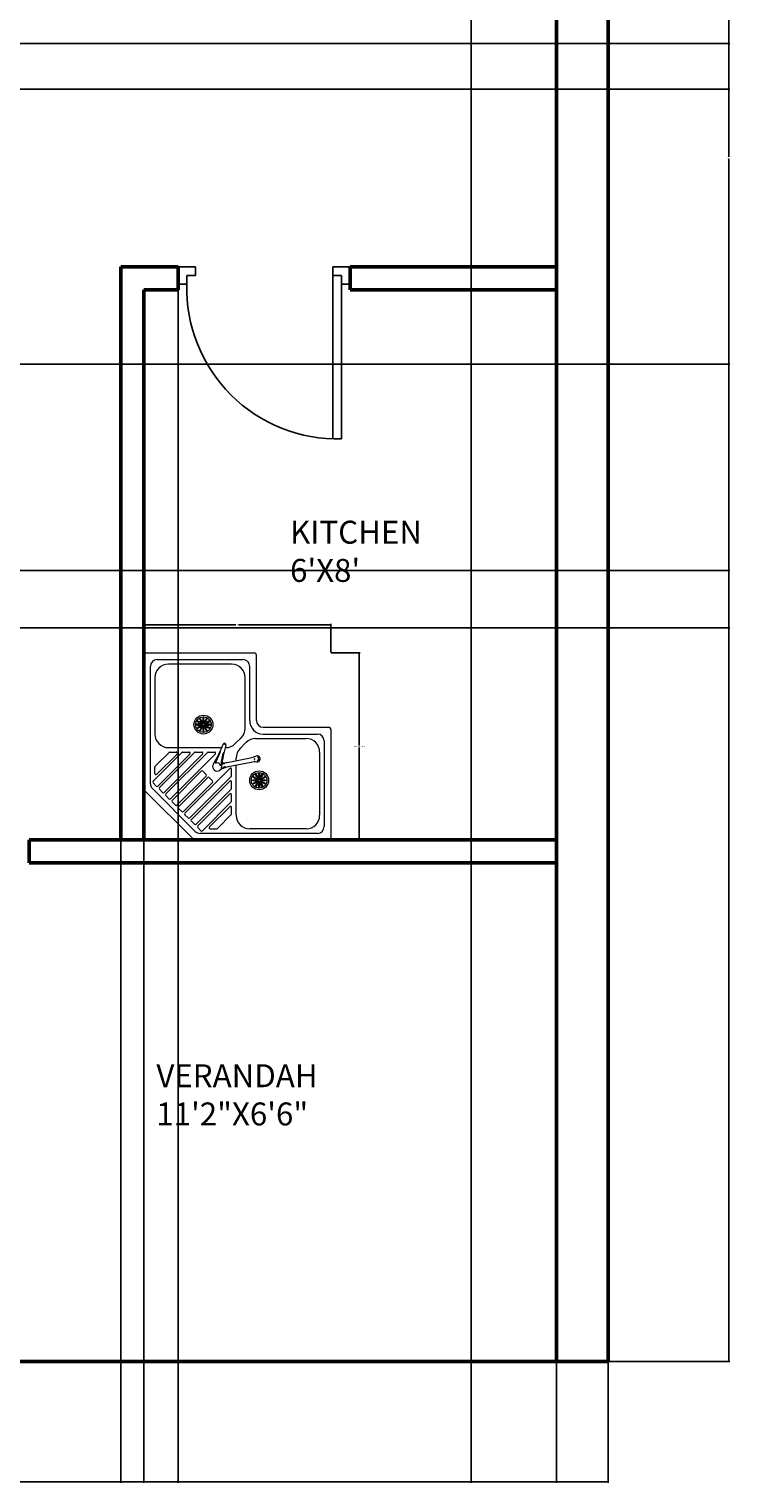
# Model space of a CAD drawing. Units: inches. Extents: x 1798 to 2141, y 1923 to 2386.
# Tile 4 of 9: x 2019 to 2141, y 1923 to 2177. Entities that reach past the tile are written whole.
import ezdxf

# ---------------------------------------------------------------- set-up
doc = ezdxf.new("R2010")
doc.units = ezdxf.units.IN
for name, color, linetype, lineweight in [('A-ANNO-DIMS', 2, 'Continuous', 18), ('A-AREA-IDEN', 7, 'Continuous', 25), ('A-FLOR-FIXT', 9, 'Continuous', 18), ('door', 40, 'Continuous', 25), ('wall', 4, 'Continuous', 50)]:
    doc.layers.add(name, color=color, linetype=linetype, lineweight=lineweight)
doc.styles.get("Standard").update_dxf_attribs({"font": 'arial.ttf'})
doc.dimstyles.get("Standard").update_dxf_attribs({"dimtxt": 0.18, "dimasz": 0.18, "dimexe": 0.18, "dimexo": 0.0625, "dimgap": 0.09, "dimtad": 0, "dimtih": 1, "dimtoh": 1, "dimdec": 4, "dimzin": 0, "dimdsep": 46, "dimtxsty": 'Standard', "dimcen": 0.09, "dimadec": 0, "dimazin": 0, "dimtfac": 1, "dimtdec": 4, "dimtofl": 0, "dimtmove": 0, "dimatfit": 3, "dimfxl": 1, "dimtolj": 1, "dimtzin": 0, "dimarcsym": 0})

# ---------------------------------------------------------------- blocks, each defined once
blk = doc.blocks.new('A$C4E531579')
for p, q in [((222.1, 827.1), (2.9, 607.9)), ((228.6, 791.2), (38.8, 601.4)), ((229.1, 830), (820, 830)), ((253.9, 788.2), (239.8, 774.1)), ((249.9, 800), (770, 800)), ((388.5, 660.7), (261, 788.2)), ((295.4, 780), (323.7, 780)), ((388.5, 717.2), (327.2, 778.5)), ((720, 780), (470, 780)), ((830, 820), (830, 340)), ((197.4, 731.6), (183.2, 717.5)), ((381.5, 512.2), (183.2, 710.4)), ((388.5, 547.5), (204.4, 731.6)), ((225.6, 759.9), (211.5, 745.8)), ((381.5, 568.7), (211.5, 738.7)), ((388.5, 604.1), (232.7, 759.9)), ((381.5, 625.3), (239.8, 767)), ((381.5, 681.9), (291.9, 771.5)), ((390, 713.7), (390, 685.4)), ((410, 720), (410, 483.9)), ((780, 440), (780, 720)), ((800, 770), (800, 390)), ((98.4, 632.6), (112.5, 646.8)), ((317.8, 448.5), (119.6, 646.8)), ((126.6, 660.9), (140.8, 675.1)), ((255.6, 524.9), (126.6, 653.9)), ((276.8, 546.1), (147.9, 675.1)), ((169.1, 703.4), (154.9, 689.2)), ((283.9, 553.2), (154.9, 682.1)), ((305.1, 574.4), (176.1, 703.4)), ((390, 657.1), (390, 628.8)), ((0, 10), (0, 600.9)), ((30, 60), (30, 580.1)), ((41.8, 576.1), (55.9, 590.2)), ((204.7, 448.5), (63, 590.2)), ((70.1, 604.4), (84.2, 618.5)), ((225.9, 441.5), (70.1, 597.3)), ((261.3, 448.5), (91.3, 618.5)), ((282.5, 441.5), (98.4, 625.6)), ((390, 600.6), (390, 572.3)), ((169.3, 441.5), (41.8, 569)), ((50, 534.6), (50, 506.3)), ((148.1, 448.5), (58.5, 538.1)), ((262.7, 524.9), (276.8, 539)), ((305.1, 567.3), (291, 553.2)), ((390, 544), (390, 515.7)), ((112.8, 441.5), (51.5, 502.8)), ((344.7, 353.4), (324.5, 455.5)), ((344.5, 460.1), (364.9, 357.1)), ((410, 468.8), (410, 466.1)), ((110, 420), (331.5, 420)), ((116.3, 440), (144.6, 440)), ((172.9, 440), (201.2, 440)), ((229.4, 440), (257.7, 440)), ((286, 440), (314.3, 440)), ((352.4, 420), (363.9, 420)), ((406.4, 402.4), (432.4, 376.4)), ((427.6, 423.6), (453.6, 397.6)), ((50, 110), (50, 360)), ((450, 333.9), (450, 110)), ((496.1, 380), (720, 380)), ((530, 360), (770, 360)), ((530, 330), (820, 330)), ((470, 300), (470, 60)), ((500, 300), (500, 10)), ((440, 30), (60, 30)), ((390, 50), (110, 50)), ((490, 0), (10, 0))]:
    blk.add_line(p, q)
for centre, radius in [((511.9, 565), 41.9), ((511.9, 565), 34.4), ((511.9, 565), 5.37), ((265, 318.1), 41.9), ((265, 318.1), 34.4), ((265, 318.1), 5.37)]:
    blk.add_circle(centre, radius)
for centre, radius, start, end in [((229.1, 820), 10, 90, 135), ((249.9, 770), 30, 90, 135), ((243.3, 770.5), 5, 135, 225), ((257.5, 784.7), 5, 45, 135), ((295.4, 775), 5, 90, 225), ((323.7, 775), 5, 45, 90), ((470, 720), 60, 90, 180), ((720, 720), 60, 0, 90), ((770, 770), 30, 0, 90), ((820, 820), 10, 0, 90), ((186.7, 714), 5, 135, 225), ((200.9, 728.1), 5, 45, 135), ((215, 742.2), 5, 135, 225), ((229.2, 756.4), 5, 45, 135), ((385, 713.7), 5, 0, 45), ((116, 643.3), 5, 45, 135), ((130.2, 657.4), 5, 135, 225), ((144.3, 671.5), 5, 45, 135), ((158.5, 685.7), 5, 135, 225), ((172.6, 699.8), 5, 45, 135), ((385, 685.4), 5, 225, 0), ((385, 657.1), 5, 0, 45), ((10, 600.9), 10, 135, 180), ((60, 580.1), 30, 135, 180), ((59.5, 586.7), 5, 45, 135), ((73.6, 600.8), 5, 135, 225), ((87.8, 615), 5, 45, 135), ((101.9, 629.1), 5, 135, 225), ((385, 628.8), 5, 225, 0), ((385, 600.6), 5, 0, 45), ((45.3, 572.5), 5, 135, 225), ((55, 534.6), 5, 45, 180), ((259.2, 528.4), 5, 225, 315), ((273.3, 542.6), 5, 315, 45), ((287.4, 556.7), 5, 225, 315), ((301.6, 570.8), 5, 315, 45), ((325.6, 504.4), 20, 52.72293, 268.78568), ((583, 916.9), 466.4, 238.27092, 250.20216), ((385, 572.3), 5, 225, 0), ((385, 515.7), 5, 225, 0), ((385, 544), 5, 0, 45), ((55, 506.3), 5, 180, 225), ((226.1, 437.3), 100, 10.4867, 33.97381), ((296.1, 462.7), 29.3, 9.84672, 38.35374), ((282.9, 16.5), 469.7, 72.94476, 84.83287), ((326.2, 504.9), 16.2, 278.92915, 32.15573), ((305.7, 211.8), 277.4, 72.23491, 84.23498), ((368.8, 476.8), 29.3, 168.25085, 191.99309), ((479.5, 750.1), 274.6, 239.9645, 252.02573), ((442.8, 478.3), 100, 177.65932, 190.48676), ((470, 466.1), 60, 180, 225), ((422.7, 471.9), 6.64, 252.6444, 68.86421), ((420.8, 471.6), 4.91, 314.25167, 37.23492), ((110, 360), 60, 90, 180), ((116.3, 445), 5, 225, 270), ((144.6, 445), 5, 270, 45), ((172.9, 445), 5, 225, 270), ((201.2, 445), 5, 270, 45), ((229.4, 445), 5, 225, 270), ((257.7, 445), 5, 270, 45), ((286, 445), 5, 225, 270), ((314.3, 445), 5, 270, 45), ((363.9, 360), 60, 45, 90), ((496.1, 440), 60, 225, 270), ((720, 440), 60, 270, 0), ((770, 390), 30, 270, 0), ((246.4, 335.2), 100, 355.98426, 10.4867), ((360, 327.2), 13.9, 175.98426, 24.98921), ((359.8, 327.5), 8.12, 180.36355, 342.44433), ((359, 332), 7.59, 72.42297, 131.67578), ((463.2, 375.3), 100, 190.48676, 204.98921), ((390, 333.9), 60, 0, 45), ((530, 300), 60, 90, 180), ((530, 300), 30, 90, 180), ((820, 340), 10, 270, 0), ((110, 110), 60, 180, 270), ((390, 110), 60, 270, 0), ((10, 10), 10, 180, 270), ((60, 60), 30, 180, 270), ((440, 60), 30, 270, 0), ((490, 10), 10, 270, 0)]:
    blk.add_arc(centre, radius, start, end)
at = {"extrusion": (-1e-16, -2e-16, -1)}
blk.add_ellipse((494.7, 574.9), major_axis=(12.6, -7.2), ratio=0.137964, dxfattribs=at)
at = {"extrusion": (0, 0, -1)}
for centre, major_axis in [((501.9, 582.2), (7.2, -12.6)), ((511.9, 584.9), (0, -14.5)), ((521.8, 547.8), (-7.2, 12.6))]:
    blk.add_ellipse(centre, major_axis=major_axis, ratio=0.137964, dxfattribs=at)
at = {"extrusion": (3e-16, -1e-16, -1)}
blk.add_ellipse((521.8, 582.2), major_axis=(-7.2, -12.6), ratio=0.137964, dxfattribs=at)
at = {"extrusion": (0, -2e-16, -1)}
for centre, major_axis in [((529.1, 574.9), (-12.6, -7.2)), ((494.7, 555.1), (12.6, 7.2))]:
    blk.add_ellipse(centre, major_axis=major_axis, ratio=0.137964, dxfattribs=at)
at = {"extrusion": (0, -1e-16, -1)}
for centre, major_axis in [((492, 565), (14.5, 0)), ((511.9, 545.1), (0, 14.5))]:
    blk.add_ellipse(centre, major_axis=major_axis, ratio=0.137964, dxfattribs=at)
at = {"extrusion": (-3e-16, 1e-16, -1)}
blk.add_ellipse((501.9, 547.8), major_axis=(7.2, 12.6), ratio=0.137964, dxfattribs=at)
at = {"extrusion": (-1e-16, -1e-16, -1)}
blk.add_ellipse((529.1, 555.1), major_axis=(-12.6, 7.2), ratio=0.137964, dxfattribs=at)
at = {"extrusion": (1e-16, -1e-16, -1)}
blk.add_ellipse((531.7, 565), major_axis=(-14.5, 0), ratio=0.137964, dxfattribs=at)
for centre, major_axis in [((247.8, 328.1), (12.6, -7.2)), ((255.1, 335.3), (7.2, -12.6)), ((265, 338), (0, -14.5)), ((274.9, 335.3), (-7.2, -12.6)), ((282.2, 328.1), (-12.6, -7.2)), ((245.1, 318.1), (14.5, 0)), ((247.8, 308.2), (12.6, 7.2)), ((255.1, 300.9), (7.2, 12.6)), ((265, 298.3), (0, 14.5)), ((274.9, 300.9), (-7.2, 12.6)), ((282.2, 308.2), (-12.6, 7.2)), ((284.9, 318.1), (-14.5, 0))]:
    blk.add_ellipse(centre, major_axis=major_axis, ratio=0.137964)
blk = doc.blocks.new('DOOR-SWING-30IN')
for p, q in [((3, 30), (0, 30)), ((0, 30), (0, 27)), ((1.5, 27), (1.5, 28.5)), ((1.5, 28.5), (3, 28.5)), ((1.5, 28.5), (30, 28.5)), ((3, 28.5), (3, 30)), ((0, 27), (1.5, 27)), ((0, 27), (30, 27)), ((0, 0), (0, 3)), ((0, 3), (1.5, 3)), ((1.5, 3), (1.5, 1.5)), ((3, 0), (0, 0)), ((1.5, 1.5), (3, 1.5)), ((3, 1.5), (3, 0))]:
    blk.add_line(p, q)
blk.add_arc((3.75, 27.75), 26.26, 268.3634, 1.6366)
blk = doc.blocks.new('*D29')
at = {"layer": 'A-ANNO-DIMS', "color": 0, "lineweight": -2, "transparency": 16777216}
for p, q in [((2071.22, 2067.97), (2076.24, 2067.97)), ((2076.06, 2067.79), (2076.06, 2051.82)), ((2076.06, 2035.47), (2076.06, 2051.45)), ((2071.22, 2035.29), (2076.24, 2035.29))]:
    blk.add_line(p, q, dxfattribs=at)
at = {"layer": 'A-ANNO-DIMS', "color": 0, "transparency": 16777216}
for points in [[(2076.03, 2067.79), (2076.09, 2067.79), (2076.06, 2067.97)], [(2076.03, 2035.47), (2076.09, 2035.47), (2076.06, 2035.29)]]:
    blk.add_solid(points, dxfattribs=at)
at = {"layer": 'Defpoints', "color": 0, "transparency": 16777216}
for p in [(2071.16, 2067.97), (2076.06, 2067.97), (2071.16, 2035.29)]:
    blk.add_point(p, dxfattribs=at)
at = {"layer": 'A-ANNO-DIMS', "color": 0, "transparency": 16777216, "insert": (2076.06, 2051.63), "char_height": 0.18, "attachment_point": 5}
blk.add_mtext('\\A1;KITCHEN SINK 33', dxfattribs=at)
blk = doc.blocks.new('*D30')
at = {"layer": 'A-ANNO-DIMS', "color": 0, "lineweight": -2, "transparency": 16777216}
for p, q in [((2038.48, 2068.03), (2038.48, 2073.05)), ((2038.66, 2072.87), (2054.6, 2072.87)), ((2070.98, 2072.87), (2055.04, 2072.87)), ((2071.16, 2068.03), (2071.16, 2073.05))]:
    blk.add_line(p, q, dxfattribs=at)
at = {"layer": 'A-ANNO-DIMS', "color": 0, "transparency": 16777216}
for points in [[(2038.66, 2072.9), (2038.66, 2072.84), (2038.48, 2072.87)], [(2070.98, 2072.9), (2070.98, 2072.84), (2071.16, 2072.87)]]:
    blk.add_solid(points, dxfattribs=at)
at = {"layer": 'Defpoints', "color": 0, "transparency": 16777216}
for p in [(2038.48, 2072.87), (2038.48, 2067.97), (2071.16, 2067.97)]:
    blk.add_point(p, dxfattribs=at)
at = {"layer": 'A-ANNO-DIMS', "color": 0, "transparency": 16777216, "insert": (2054.82, 2072.87), "char_height": 0.18, "attachment_point": 5}
blk.add_mtext('\\A1;33', dxfattribs=at)
blk = doc.blocks.new('*D31')
at = {"layer": 'A-ANNO-DIMS', "color": 0, "lineweight": -2, "transparency": 16777216}
for p, q in [((1819.51, 1944.26), (1819.51, 1923.12)), ((2119.51, 1944.26), (2119.51, 1923.12)), ((1819.69, 1923.3), (1969.23, 1923.3)), ((2119.33, 1923.3), (1969.8, 1923.3))]:
    blk.add_line(p, q, dxfattribs=at)
at = {"layer": 'A-ANNO-DIMS', "color": 0, "transparency": 16777216}
for points in [[(1819.69, 1923.33), (1819.69, 1923.27), (1819.51, 1923.3)], [(2119.33, 1923.33), (2119.33, 1923.27), (2119.51, 1923.3)]]:
    blk.add_solid(points, dxfattribs=at)
at = {"layer": 'Defpoints', "color": 0, "transparency": 16777216}
for p in [(1819.51, 1944.32), (2119.51, 1944.32), (2119.51, 1923.3)]:
    blk.add_point(p, dxfattribs=at)
at = {"layer": 'A-ANNO-DIMS', "color": 0, "transparency": 16777216, "insert": (1969.51, 1923.3), "char_height": 0.18, "attachment_point": 5}
blk.add_mtext('\\A1;300', dxfattribs=at)
blk = doc.blocks.new('*D32')
at = {"layer": 'A-ANNO-DIMS', "color": 0, "lineweight": -2, "transparency": 16777216}
for p, q in [((2119.58, 2364.32), (2140.72, 2364.32)), ((2140.54, 2364.14), (2140.54, 2154.51)), ((2140.54, 1944.5), (2140.54, 2154.14)), ((2119.58, 1944.32), (2140.72, 1944.32))]:
    blk.add_line(p, q, dxfattribs=at)
at = {"layer": 'A-ANNO-DIMS', "color": 0, "transparency": 16777216}
for points in [[(2140.51, 2364.14), (2140.57, 2364.14), (2140.54, 2364.32)], [(2140.51, 1944.5), (2140.57, 1944.5), (2140.54, 1944.32)]]:
    blk.add_solid(points, dxfattribs=at)
at = {"layer": 'Defpoints', "color": 0, "transparency": 16777216}
for p in [(2119.51, 2364.32), (2140.54, 2364.32), (2119.51, 1944.32)]:
    blk.add_point(p, dxfattribs=at)
at = {"layer": 'A-ANNO-DIMS', "color": 0, "transparency": 16777216, "insert": (2140.54, 2154.32), "char_height": 0.18, "attachment_point": 5}
blk.add_mtext('\\A1;420', dxfattribs=at)
blk = doc.blocks.new('*D38')
at = {"layer": 'A-ANNO-DIMS', "color": 0, "lineweight": -2, "transparency": 16777216}
for p, q in [((2038.51, 2131.26), (2038.51, 1923.12)), ((2044.51, 2131.26), (2044.51, 1923.12)), ((2038.69, 1923.3), (2041.36, 1923.3)), ((2044.33, 1923.3), (2041.66, 1923.3))]:
    blk.add_line(p, q, dxfattribs=at)
at = {"layer": 'A-ANNO-DIMS', "color": 0, "transparency": 16777216}
for points in [[(2038.69, 1923.33), (2038.69, 1923.27), (2038.51, 1923.3)], [(2044.33, 1923.33), (2044.33, 1923.27), (2044.51, 1923.3)]]:
    blk.add_solid(points, dxfattribs=at)
at = {"layer": 'Defpoints', "color": 0, "transparency": 16777216}
for p in [(2038.51, 2131.32), (2044.51, 2131.32), (2044.51, 1923.3)]:
    blk.add_point(p, dxfattribs=at)
at = {"layer": 'A-ANNO-DIMS', "color": 0, "transparency": 16777216, "insert": (2041.51, 1923.3), "char_height": 0.18, "attachment_point": 5}
blk.add_mtext('\\A1;6', dxfattribs=at)
blk = doc.blocks.new('*D40')
at = {"layer": 'A-ANNO-DIMS', "color": 0, "lineweight": -2, "transparency": 16777216}
for p, q in [((1976.58, 2082.32), (2140.72, 2082.32)), ((2140.54, 2082.14), (2140.54, 2077.51)), ((2140.54, 2072.5), (2140.54, 2077.14)), ((1976.58, 2072.32), (2140.72, 2072.32))]:
    blk.add_line(p, q, dxfattribs=at)
at = {"layer": 'A-ANNO-DIMS', "color": 0, "transparency": 16777216}
for points in [[(2140.51, 2082.14), (2140.57, 2082.14), (2140.54, 2082.32)], [(2140.51, 2072.5), (2140.57, 2072.5), (2140.54, 2072.32)]]:
    blk.add_solid(points, dxfattribs=at)
at = {"layer": 'Defpoints', "color": 0, "transparency": 16777216}
for p in [(1976.51, 2082.32), (2140.54, 2082.32), (1976.51, 2072.32)]:
    blk.add_point(p, dxfattribs=at)
at = {"layer": 'A-ANNO-DIMS', "color": 0, "transparency": 16777216, "insert": (2140.54, 2077.32), "char_height": 0.18, "attachment_point": 5}
blk.add_mtext('\\A1;10', dxfattribs=at)
blk = doc.blocks.new('*D44')
at = {"layer": 'A-ANNO-DIMS', "color": 0, "lineweight": -2, "transparency": 16777216}
for p, q in [((1920.58, 2118.32), (2140.72, 2118.32)), ((2140.54, 2118.14), (2140.54, 2100.51)), ((2140.54, 2082.5), (2140.54, 2100.14)), ((1920.58, 2082.32), (2140.72, 2082.32))]:
    blk.add_line(p, q, dxfattribs=at)
at = {"layer": 'A-ANNO-DIMS', "color": 0, "transparency": 16777216}
for points in [[(2140.51, 2118.14), (2140.57, 2118.14), (2140.54, 2118.32)], [(2140.51, 2082.5), (2140.57, 2082.5), (2140.54, 2082.32)]]:
    blk.add_solid(points, dxfattribs=at)
at = {"layer": 'Defpoints', "color": 0, "transparency": 16777216}
for p in [(1920.51, 2118.32), (1920.51, 2082.32), (2140.54, 2082.32)]:
    blk.add_point(p, dxfattribs=at)
at = {"layer": 'A-ANNO-DIMS', "color": 0, "transparency": 16777216, "insert": (2140.54, 2100.32), "char_height": 0.18, "attachment_point": 5}
blk.add_mtext('\\A1;36', dxfattribs=at)
blk = doc.blocks.new('*D45')
at = {"layer": 'A-ANNO-DIMS', "color": 0, "lineweight": -2, "transparency": 16777216}
for p, q in [((1864.58, 2174.32), (2140.72, 2174.32)), ((2140.54, 2174.14), (2140.54, 2170.51)), ((2140.54, 2166.5), (2140.54, 2170.14)), ((1864.58, 2166.32), (2140.72, 2166.32))]:
    blk.add_line(p, q, dxfattribs=at)
at = {"layer": 'A-ANNO-DIMS', "color": 0, "transparency": 16777216}
for points in [[(2140.51, 2174.14), (2140.57, 2174.14), (2140.54, 2174.32)], [(2140.51, 2166.5), (2140.57, 2166.5), (2140.54, 2166.32)]]:
    blk.add_solid(points, dxfattribs=at)
at = {"layer": 'Defpoints', "color": 0, "transparency": 16777216}
for p in [(1864.51, 2174.32), (2140.54, 2174.32), (1864.51, 2166.32)]:
    blk.add_point(p, dxfattribs=at)
at = {"layer": 'A-ANNO-DIMS', "color": 0, "transparency": 16777216, "insert": (2140.54, 2170.32), "char_height": 0.18, "attachment_point": 5}
blk.add_mtext('\\A1;8', dxfattribs=at)
blk = doc.blocks.new('*D46')
at = {"layer": 'A-ANNO-DIMS', "color": 0, "lineweight": -2, "transparency": 16777216}
for p, q in [((1982.72, 2148.29), (1982.72, 1923.12)), ((2034.51, 2135.26), (2034.51, 1923.12)), ((1982.9, 1923.3), (2008.22, 1923.3)), ((2034.33, 1923.3), (2009.01, 1923.3))]:
    blk.add_line(p, q, dxfattribs=at)
at = {"layer": 'A-ANNO-DIMS', "color": 0, "transparency": 16777216}
for points in [[(1982.9, 1923.33), (1982.9, 1923.27), (1982.72, 1923.3)], [(2034.33, 1923.33), (2034.33, 1923.27), (2034.51, 1923.3)]]:
    blk.add_solid(points, dxfattribs=at)
at = {"layer": 'Defpoints', "color": 0, "transparency": 16777216}
for p in [(1982.72, 2148.35), (2034.51, 2135.32), (2034.51, 1923.3)]:
    blk.add_point(p, dxfattribs=at)
at = {"layer": 'A-ANNO-DIMS', "color": 0, "transparency": 16777216, "insert": (2008.62, 1923.3), "char_height": 0.18, "attachment_point": 5}
blk.add_mtext('\\A1;51.79', dxfattribs=at)
blk = doc.blocks.new('*D48')
at = {"layer": 'A-ANNO-DIMS', "color": 0, "lineweight": -2, "transparency": 16777216}
for p, q in [((2095.64, 2183.26), (2095.64, 1923.12)), ((2110.51, 2183.26), (2110.51, 1923.12)), ((2095.82, 1923.3), (2102.62, 1923.3)), ((2110.33, 1923.3), (2103.53, 1923.3))]:
    blk.add_line(p, q, dxfattribs=at)
at = {"layer": 'A-ANNO-DIMS', "color": 0, "transparency": 16777216}
for points in [[(2095.82, 1923.33), (2095.82, 1923.27), (2095.64, 1923.3)], [(2110.33, 1923.33), (2110.33, 1923.27), (2110.51, 1923.3)]]:
    blk.add_solid(points, dxfattribs=at)
at = {"layer": 'Defpoints', "color": 0, "transparency": 16777216}
for p in [(2095.64, 2183.32), (2110.51, 2183.32), (2110.51, 1923.3)]:
    blk.add_point(p, dxfattribs=at)
at = {"layer": 'A-ANNO-DIMS', "color": 0, "transparency": 16777216, "insert": (2103.08, 1923.3), "char_height": 0.18, "attachment_point": 5}
blk.add_mtext('\\A1;14.878', dxfattribs=at)

msp = doc.modelspace()

# ---------------------------------------------------------------- linework, layer by layer
at = {"layer": 'wall'}
for p, q in [((2119.5141, 1944.3239), (2119.5141, 2364.3239)), ((2110.5141, 1944.3239), (2110.5141, 2355.3239)), ((2034.5141, 2035.3239), (2034.5141, 2135.3239)), ((2038.5141, 2135.3239), (2034.5141, 2135.3239)), ((2044.5141, 2135.3239), (2038.5141, 2135.3239)), ((2044.5141, 2131.3239), (2044.5141, 2135.3239)), ((2110.5141, 2135.3239), (2074.5141, 2135.3239)), ((2074.5141, 2131.3239), (2074.5141, 2135.3239)), ((2038.5141, 2035.3239), (2038.5141, 2131.3239)), ((2044.5141, 2131.3239), (2038.5141, 2131.3239)), ((2110.5141, 2131.3239), (2074.5141, 2131.3239)), ((2034.5141, 2035.3239), (2034.5141, 2082.3239)), ((2038.5141, 2035.3239), (2038.5141, 2082.3239)), ((2110.5141, 2035.3239), (2018.5141, 2035.3239)), ((2018.5141, 2035.3239), (2018.5141, 2031.3239)), ((2110.5141, 2031.3239), (2018.5141, 2031.3239)), ((1819.5141, 1944.3239), (2119.5141, 1944.3239))]:
    msp.add_line(p, q, dxfattribs=at)

# ---------------------------------------------------------------- block references
at = {"layer": 'A-FLOR-FIXT', "xscale": 0.0393700787401575, "yscale": 0.0393700787401575, "zscale": 0.0393700787401575, "rotation": 90}
msp.add_blockref('A$C4E531579', (2071.1613, 2035.2939), dxfattribs=at)
at = {"layer": 'door', "rotation": 270.0000000000023}
msp.add_blockref('DOOR-SWING-30IN', (2044.5141, 2135.3239), dxfattribs=at)

# ---------------------------------------------------------------- texts
at = {"layer": 'A-AREA-IDEN', "char_height": 4, "attachment_point": 1}
for s, insert in [("\\pxt7;KITCHEN\\P6'X8'", (2064.0303, 2091.0244)), ('VERANDAH\\P11\'2"X6\'6"', (2040.7094, 1996.1734))]:
    msp.add_mtext_dynamic_manual_height_columns(s, width=35.513916, gutter_width=12.5, heights=[0], dxfattribs=dict(at, insert=insert))

# ---------------------------------------------------------------- dimensions: what is measured, and where the dimension line sits
at = {"layer": 'A-ANNO-DIMS'}
for base, p1, p2, angle, picture, middle in [((2140.5391, 2364.3239), (2119.5141, 1944.3239), (2119.5141, 2364.3239), 90, '*D32', (2140.5391, 2154.3239)), ((2140.5391, 2174.3239), (1864.5141, 2166.3239), (1864.5141, 2174.3239), 90, '*D45', (2140.5391, 2170.3239)), ((2140.5391, 2082.3239), (1920.5141, 2118.3239), (1920.5141, 2082.3239), 90, '*D44', (2140.5391, 2100.3239)), ((2140.5391, 2082.3239), (1976.5141, 2072.3239), (1976.5141, 2082.3239), 90, '*D40', (2140.5391, 2077.3239)), ((2038.4841, 2072.8727), (2071.1613, 2067.9711), (2038.4841, 2067.9711), 180, '*D30', (2054.8227, 2072.8727))]:
    dim = msp.add_linear_dim(base=base, p1=p1, p2=p2, angle=angle, dimstyle='Standard', override={"dimdec": 0, "dimlfac": 1, "dimrnd": 0, "dimzin": 0, "dimdsep": 46, "dimlunit": 2}, dxfattribs=at)
    dim.commit()
    dim.dimension.update_dxf_attribs({"geometry": picture, "text_midpoint": middle})
for base, p1, p2, override, picture, middle in [((2110.5141, 1923.2989), (2095.6365, 2183.3239), (2110.5141, 2183.3239), {"dimdec": 3, "dimlfac": 1, "dimrnd": 0, "dimzin": 0, "dimdsep": 46, "dimlunit": 2}, '*D48', (2103.0753, 1923.2989)), ((2034.5141, 1923.2989), (1982.7222, 2148.3502), (2034.5141, 2135.3239), {"dimdec": 2, "dimlfac": 1, "dimrnd": 0, "dimzin": 0, "dimdsep": 46, "dimlunit": 2}, '*D46', (2008.6182, 1923.2989)), ((2044.5141, 1923.2989), (2038.5141, 2131.3239), (2044.5141, 2131.3239), {"dimdec": 0, "dimlfac": 1, "dimrnd": 0, "dimzin": 0, "dimdsep": 46, "dimlunit": 2}, '*D38', (2041.5141, 1923.2989)), ((2119.5141, 1923.2989), (1819.5141, 1944.3239), (2119.5141, 1944.3239), {"dimdec": 0, "dimlfac": 1, "dimrnd": 0, "dimzin": 0, "dimdsep": 46, "dimlunit": 2}, '*D31', (1969.5141, 1923.2989))]:
    dim = msp.add_linear_dim(base=base, p1=p1, p2=p2, dimstyle='Standard', override=override, dxfattribs=at)
    dim.commit()
    dim.dimension.update_dxf_attribs({"geometry": picture, "text_midpoint": middle})
dim = msp.add_linear_dim(base=(2076.0629, 2067.9711), p1=(2071.1613, 2035.2939), p2=(2071.1613, 2067.9711), angle=90, text='KITCHEN SINK <>', dimstyle='Standard', override={"dimdec": 0, "dimlfac": 1, "dimrnd": 0, "dimzin": 0, "dimdsep": 46, "dimlunit": 2}, dxfattribs=at)
dim.commit()
dim.dimension.update_dxf_attribs({"geometry": '*D29', "text_midpoint": (2076.0629, 2051.6325)})

doc.saveas('drawing.dxf')
